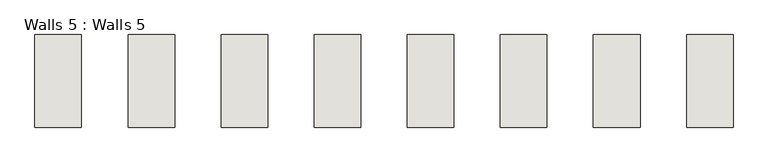
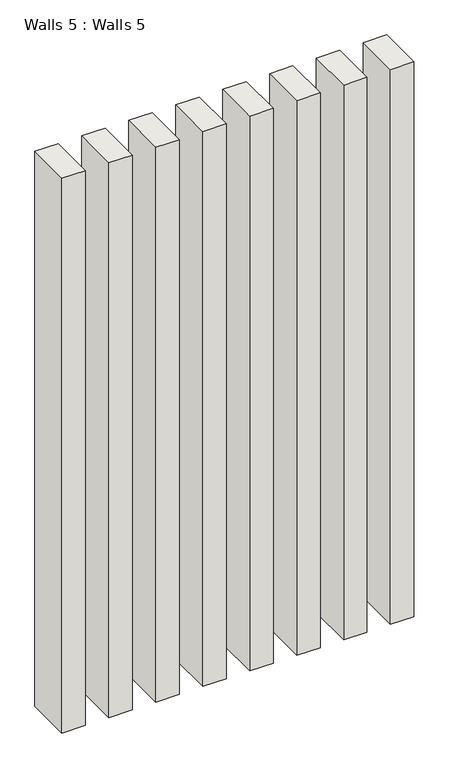
"""IFC4 building model written with IfcOpenShell, lengths in millimetres: wall geometry, Walls 5 : Walls 5."""

from ifc_helpers import new_model, si_unit, frame, origin, place, context, project, spatial, polyline, outline, extrude, source, transform, mapped, element, save


def walls_5_walls_5_96d48458(model_context):
    return source(origin(), model_context, "Body", "SweptSolid", [
        extrude(outline(polyline([(7121.577479, -16160.3467593), (6969.177479, -16160.3467593), (6969.177479, -15855.5467593), (7121.577479, -15855.5467593), (7121.577479, -16160.3467593)])), frame((0.0, 0.0, 2895.6), z_axis=(0.0, 0.0, 1.0), x_axis=(1.0, 0.0, 0.0)), (0.0, 0.0, 1.0), 3810.0),
        extrude(outline(polyline([(7426.377479, -16160.3467593), (7273.977479, -16160.3467593), (7273.977479, -15855.5467593), (7426.377479, -15855.5467593), (7426.377479, -16160.3467593)])), frame((0.0, 0.0, 2895.6), z_axis=(0.0, 0.0, 1.0), x_axis=(1.0, 0.0, 0.0)), (0.0, 0.0, 1.0), 3810.0),
        extrude(outline(polyline([(7731.177479, -16160.3467593), (7578.777479, -16160.3467593), (7578.777479, -15855.5467593), (7731.177479, -15855.5467593), (7731.177479, -16160.3467593)])), frame((0.0, 0.0, 2895.6), z_axis=(0.0, 0.0, 1.0), x_axis=(1.0, 0.0, 0.0)), (0.0, 0.0, 1.0), 3810.0),
        extrude(outline(polyline([(8035.977479, -16160.3467593), (7883.577479, -16160.3467593), (7883.577479, -15855.5467593), (8035.977479, -15855.5467593), (8035.977479, -16160.3467593)])), frame((0.0, 0.0, 2895.6), z_axis=(0.0, 0.0, 1.0), x_axis=(1.0, 0.0, 0.0)), (0.0, 0.0, 1.0), 3810.0),
        extrude(outline(polyline([(8340.777479, -16160.3467593), (8188.377479, -16160.3467593), (8188.377479, -15855.5467593), (8340.777479, -15855.5467593), (8340.777479, -16160.3467593)])), frame((0.0, 0.0, 2895.6), z_axis=(0.0, 0.0, 1.0), x_axis=(1.0, 0.0, 0.0)), (0.0, 0.0, 1.0), 3810.0),
        extrude(outline(polyline([(8645.577479, -16160.3467593), (8493.177479, -16160.3467593), (8493.177479, -15855.5467593), (8645.577479, -15855.5467593), (8645.577479, -16160.3467593)])), frame((0.0, 0.0, 2895.6), z_axis=(0.0, 0.0, 1.0), x_axis=(1.0, 0.0, 0.0)), (0.0, 0.0, 1.0), 3810.0),
        extrude(outline(polyline([(8950.377479, -16160.3467593), (8797.977479, -16160.3467593), (8797.977479, -15855.5467593), (8950.377479, -15855.5467593), (8950.377479, -16160.3467593)])), frame((0.0, 0.0, 2895.6), z_axis=(0.0, 0.0, 1.0), x_axis=(1.0, 0.0, 0.0)), (0.0, 0.0, 1.0), 3810.0),
        extrude(outline(polyline([(9255.177479, -16160.3467593), (9102.777479, -16160.3467593), (9102.777479, -15855.5467593), (9255.177479, -15855.5467593), (9255.177479, -16160.3467593)])), frame((0.0, 0.0, 2895.6), z_axis=(0.0, 0.0, 1.0), x_axis=(1.0, 0.0, 0.0)), (0.0, 0.0, 1.0), 3810.0),
    ])


if __name__ == "__main__":
    model = new_model("IFC4")
    model_context = context("Model", 3, world=origin())
    ifc_project = project(units=[si_unit("LENGTHUNIT", "METRE", prefix="MILLI")], contexts=[model_context])
    site = spatial("IfcSite", under=ifc_project)
    building = spatial("IfcBuilding", under=site)
    placement = place(None, origin())
    walls_5_walls_5_shape = walls_5_walls_5_96d48458(model_context)
    element("IfcWall", 1, ObjectType="Walls 5 : Walls 5", at=placement, inside=building, context=model_context, shape_type="MappedRepresentation", body=[
        mapped(walls_5_walls_5_shape, transform((0.0, 0.0, 0.0), x_axis=(1.0, 0.0, 0.0), y_axis=(0.0, 1.0, 0.0), z_axis=(0.0, 0.0, 1.0))),
    ])
    save(model, "model.ifc")

# Revit data of these elements
# Element 1 (IfcWall, "Walls 5 : Walls 5")
#   Materials on its faces: "Sash", "Default Wall"
# Materials
#   "Sash": class "Wood", colour RGB 224 178 126, transparency 0
#   "Default Wall": colour RGB 128 128 128, transparency 0
